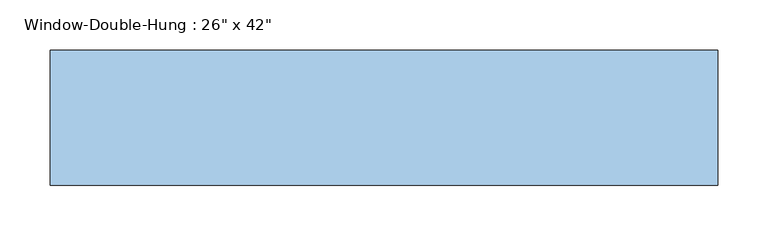
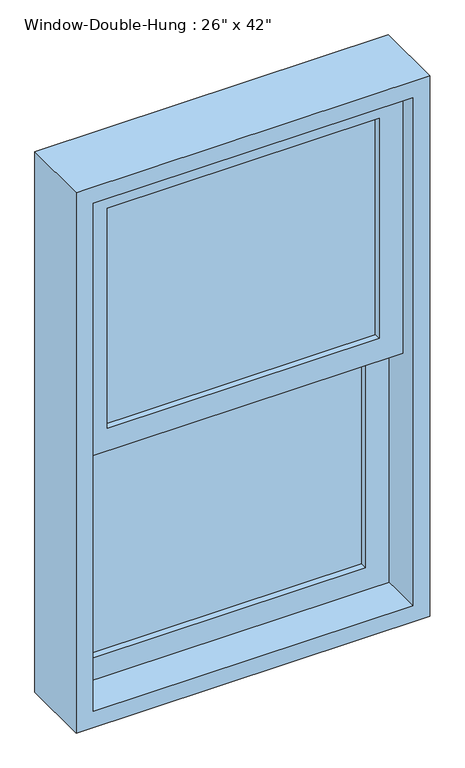
"""IFC4 building model written with IfcOpenShell, lengths in millimetres: window geometry."""

from ifc_helpers import new_model, si_unit, frame, origin, place, context, project, spatial, polyline, outline, extrude, source, transform, mapped, element, save


def window_d2058a86(model_context):
    return source(origin(), model_context, "Body", "SweptSolid", [
        extrude(outline(polyline([(254.0, 12.7), (-254.0, 12.7), (-254.0, 19.05), (254.0, 19.05), (254.0, 12.7)])), frame((0.0, 0.0, 990.6), z_axis=(0.0, 0.0, 1.0), x_axis=(1.0, 0.0, 0.0)), (0.0, 0.0, 1.0), 434.975),
        extrude(outline(polyline([(-254.0, 25.4), (-254.0, 31.75), (254.0, 31.75), (254.0, 25.4), (-254.0, 25.4)])), frame((0.0, 0.0, 990.6), z_axis=(0.0, 0.0, 1.0), x_axis=(1.0, 0.0, 0.0)), (0.0, 0.0, 1.0), 434.975),
        extrude(outline(polyline([(254.0, -31.75), (-254.0, -31.75), (-254.0, -25.4), (254.0, -25.4), (254.0, -31.75)])), frame((0.0, 0.0, 1470.025), z_axis=(0.0, 0.0, 1.0), x_axis=(1.0, 0.0, 0.0)), (0.0, 0.0, 1.0), 434.975),
        extrude(outline(polyline([(-254.0, -19.05), (-254.0, -12.7), (254.0, -12.7), (254.0, -19.05), (-254.0, -19.05)])), frame((0.0, 0.0, 1470.025), z_axis=(0.0, 0.0, 1.0), x_axis=(1.0, 0.0, 0.0)), (0.0, 0.0, 1.0), 434.975),
        extrude(outline(polyline([(1470.025, 298.45), (1470.025, -298.45), (946.15, -298.45), (946.15, 298.45), (1470.025, 298.45)]), holes=[polyline([(1425.575, -254.0), (1425.575, 254.0), (990.6, 254.0), (990.6, -254.0), (1425.575, -254.0)])]), frame((0.0, 0.0, 0.0), z_axis=(0.0, 1.0, 0.0), x_axis=(0.0, 0.0, 1.0)), (0.0, 0.0, 1.0), 44.45),
        extrude(outline(polyline([(1949.45, 298.45), (1949.45, -298.45), (1425.575, -298.45), (1425.575, 298.45), (1949.45, 298.45)]), holes=[polyline([(1905.0, -254.0), (1905.0, 254.0), (1470.025, 254.0), (1470.025, -254.0), (1905.0, -254.0)])]), frame((0.0, -44.45, 0.0), z_axis=(0.0, 1.0, 0.0), x_axis=(0.0, 0.0, 1.0)), (0.0, 0.0, 1.0), 44.45),
        extrude(outline(polyline([(1981.2, 330.2), (1981.2, -330.2), (914.4, -330.2), (914.4, 330.2), (1981.2, 330.2)]), holes=[polyline([(1949.45, -298.45), (1949.45, 298.45), (946.15, 298.45), (946.15, -298.45), (1949.45, -298.45)])]), frame((0.0, -76.2, 0.0), z_axis=(0.0, 1.0, 0.0), x_axis=(0.0, 0.0, 1.0)), (0.0, 0.0, 1.0), 133.35),
    ])


if __name__ == "__main__":
    model = new_model("IFC4")
    model_context = context("Model", 3, world=origin())
    ifc_project = project(units=[si_unit("LENGTHUNIT", "METRE", prefix="MILLI")], contexts=[model_context])
    site = spatial("IfcSite", under=ifc_project)
    building = spatial("IfcBuilding", under=site)
    placement = place(None, origin())
    window_shape = window_d2058a86(model_context)
    element("IfcWindow", 1, ObjectType="Window-Double-Hung : 26\" x 42\"", at=placement, inside=building, context=model_context, shape_type="MappedRepresentation", body=[
        mapped(window_shape, transform((0.0, 0.0, 0.0), x_axis=(1.0, 0.0, 0.0), y_axis=(0.0, 1.0, 0.0), z_axis=(0.0, 0.0, 1.0))),
    ])
    save(model, "model.ifc")

# Revit data of these elements
# Type "Window-Double-Hung : 26\" x 42\""
#   Type Mark = "11"
#   Fire Rating = "0.5h"
#   Construction Type Id = "DG-DR"
#   Assembly Code = "B2020100"
#   Analytic Construction = "Double glazing - domestic"
#   Wall Thickness [instance default] = 0' - 6"
#   Window Inset [instance default] = 0' - 0"
#   Visual Light Transmittance = 0.81
#   Thermal Resistance (R) = 1.8146 (h·ft²·°F)/BTU
#   Solar Heat Gain Coefficient = 0.76
#   Muntin Width = 1' - 8"
#   Muntin Height = 1' - 5 1/8"
#   Interior Wall Closure [instance default] = 0' - 1 1/2"
#   Rough Width = 2' - 2 1/2"
#   Rough Height = 3' - 6 1/2"
#   Frame Extension [instance default] = 0' - 1 1/4"
#   Exterior Wall Closure [instance default] = 0' - 0 1/2"
#   Extension Jamb [instance default] = 0' - 1 1/2"
#   Heat Transfer Coefficient (U) = 0.5511 BTU/(h·ft²·°F)
#   Height = 3' - 6"
#   Width = 2' - 2"
#   Define Thermal Properties by = 1
#   Top Muntin Visibility = yes
#   Indicator Visibility [instance default] = yes
#   Extension Jamb Visibility [instance default] = yes
#   Interior Trim Visibility [instance default] = yes
#   Exterior Trim Visibility [instance default] = yes
#   Define Thermal Properties by = 1
#   Bottom Muntin Visibility = yes
#   Muntin Pattern = Muntin Pattern_2x2 : Muntin Pattern_2x2
#   Interior Trim Material = Wood - Stained
#   Interior Trim = Trim-Window-Interior-Flat : Picture Frame
#   Exterior Trim Material = Clad - White
#   Exterior Trim = Trim-Window-Exterior-Flat : with Sill
#   Glass Panel Material = Glass
#   Exterior Frame Material = Clad - White
#   Interior Frame Material = Wood - Stained
#   Wall Closure = (empty or 0)
# Element 1 (IfcWindow, "Window-Double-Hung : 26\" x 42\"")
#   Wall Thickness = 0' - 4 1/2"
#   Extension Jamb = 0' - 1"
#   Extension Jamb Visibility = no
#   Materials on its faces: "Wood - Stained", "Glass", "Clad - White"
# Materials
#   "Wood - Stained": class "Wood", colour RGB 224 178 126, transparency 0, Cost = 0
#   "Clad - White": class "Wood", colour RGB 242 242 238, transparency 0, Cost = 0
#   "Glass": class "Glass", colour RGB 0 128 192, transparency 0.75, Description = "Soda Lime Glass", Cost = 0
